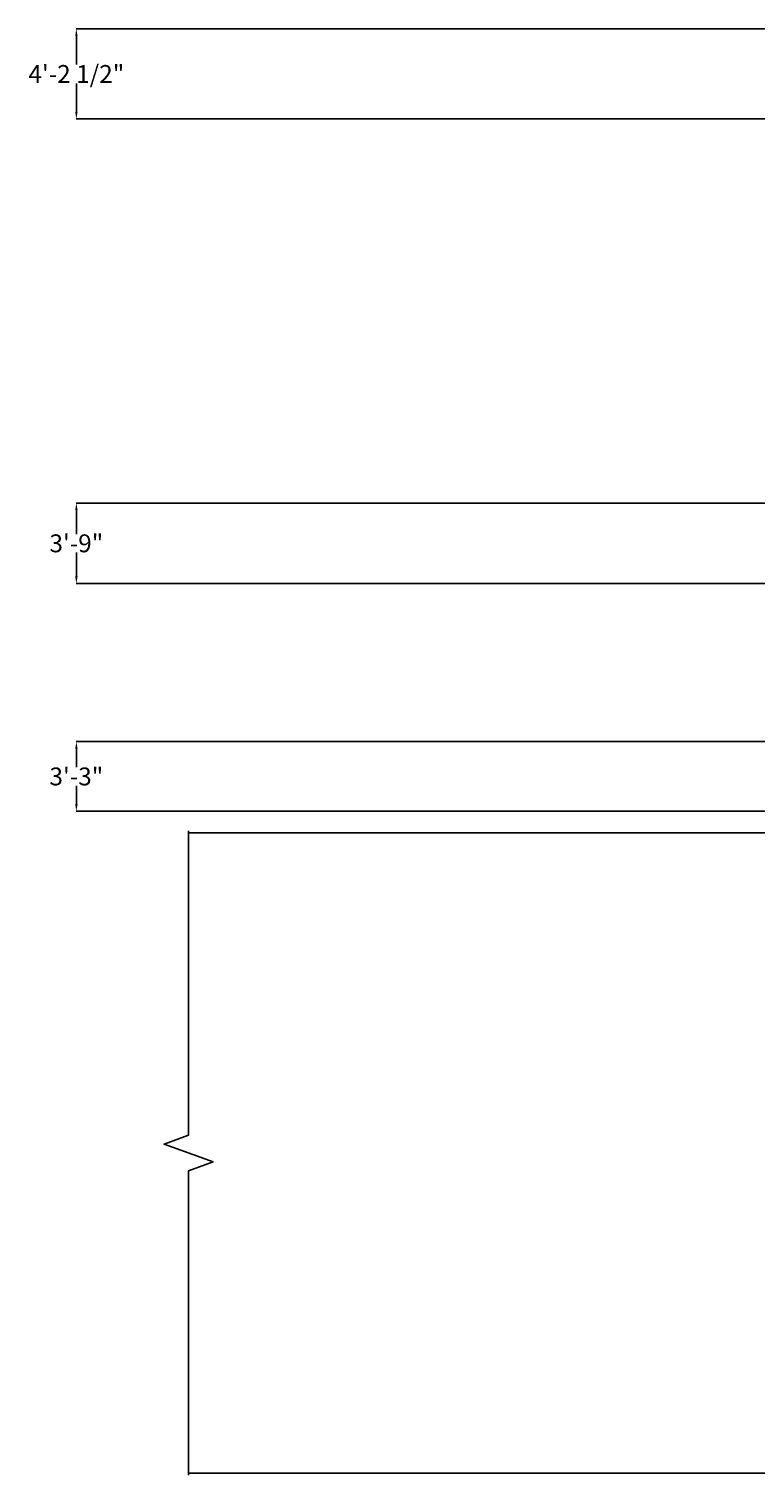
# Model space of a CAD drawing. Units: inches. Extents: x 529 to 1659, y 271 to 1222.
# Tile 1 of 5: x 529 to 936, y 326 to 1136. Entities that reach past the tile are written whole.
import ezdxf

# ---------------------------------------------------------------- set-up
doc = ezdxf.new("R2010")
doc.units = ezdxf.units.IN
doc.header["$MEASUREMENT"] = 0
doc.layers.add('C-ROAD', color=7, linetype='Continuous', lineweight=25)
doc.layers.add('DIM', color=241, linetype='Continuous', lineweight=18)
doc.styles.get("Standard").update_dxf_attribs({"font": 'arial.ttf', "height": 10})
doc.dimstyles.get("Standard").update_dxf_attribs({"dimtxt": 6, "dimasz": 4, "dimexe": 0.18, "dimexo": 0.0625, "dimgap": 0.09, "dimtad": 0, "dimtih": 1, "dimtoh": 1, "dimdec": 0, "dimrnd": 6, "dimzin": 0, "dimdsep": 46, "dimlunit": 3, "dimtxsty": 'Standard', "dimcen": 0.09, "dimadec": 0, "dimazin": 0, "dimtfac": 1, "dimtdec": 0, "dimtofl": 0, "dimtmove": 0, "dimatfit": 3, "dimfxl": 1, "dimtolj": 1, "dimtzin": 0, "dimarcsym": 0})

# ---------------------------------------------------------------- blocks, each defined once
blk = doc.blocks.new('ROAD-BREAKLINE')
blk.add_lwpolyline([(13.74, 0), (13.74, 170.31), (27.47, 175.31), (0, 185.31), (13.74, 190.31), (13.74, 360.62)])
blk = doc.blocks.new('*D32')
at = {"layer": 'Defpoints', "color": 0, "transparency": 16777216}
for p in [(555.49, 736.86), (1020.49, 736.86), (1020.49, 697.86)]:
    blk.add_point(p, dxfattribs=at)
at = {"layer": 'DIM', "color": 0, "lineweight": -2, "transparency": 16777216}
for p, q in [((1020.43, 736.86), (555.31, 736.86)), ((555.49, 732.86), (555.49, 722.55)), ((555.49, 701.86), (555.49, 712.16)), ((1020.43, 697.86), (555.31, 697.86))]:
    blk.add_line(p, q, dxfattribs=at)
at = {"layer": 'DIM', "color": 0, "transparency": 16777216}
for points in [[(554.83, 732.86), (556.16, 732.86), (555.49, 736.86)], [(554.83, 701.86), (556.16, 701.86), (555.49, 697.86)]]:
    blk.add_solid(points, dxfattribs=at)
at = {"layer": 'DIM', "color": 0, "transparency": 16777216, "insert": (555.49, 717.36), "char_height": 10, "attachment_point": 5}
blk.add_mtext('\\A1;3\'-3"', dxfattribs=at)
blk = doc.blocks.new('*D33')
at = {"layer": 'Defpoints', "color": 0, "transparency": 16777216}
for p in [(555.49, 870.44), (1020.49, 870.44), (1020.41, 825.31)]:
    blk.add_point(p, dxfattribs=at)
at = {"layer": 'DIM', "color": 0, "lineweight": -2, "transparency": 16777216}
for p, q in [((1020.43, 870.44), (555.31, 870.44)), ((555.49, 866.44), (555.49, 853.07)), ((555.49, 829.31), (555.49, 842.67)), ((1020.35, 825.31), (555.31, 825.31))]:
    blk.add_line(p, q, dxfattribs=at)
at = {"layer": 'DIM', "color": 0, "transparency": 16777216}
for points in [[(554.83, 866.44), (556.16, 866.44), (555.49, 870.44)], [(554.83, 829.31), (556.16, 829.31), (555.49, 825.31)]]:
    blk.add_solid(points, dxfattribs=at)
at = {"layer": 'DIM', "color": 0, "transparency": 16777216, "insert": (555.49, 847.87), "char_height": 10, "attachment_point": 5}
blk.add_mtext('\\A1;3\'-9"', dxfattribs=at)
blk = doc.blocks.new('*D35')
at = {"layer": 'Defpoints', "color": 0, "transparency": 16777216}
for p in [(555.49, 1135.86), (1020.49, 1135.86), (1029.49, 1085.43)]:
    blk.add_point(p, dxfattribs=at)
at = {"layer": 'DIM', "color": 0, "lineweight": -2, "transparency": 16777216}
for p, q in [((1020.43, 1135.86), (555.31, 1135.86)), ((555.49, 1131.86), (555.49, 1115.9)), ((555.49, 1089.43), (555.49, 1105.38)), ((1029.43, 1085.43), (555.31, 1085.43))]:
    blk.add_line(p, q, dxfattribs=at)
at = {"layer": 'DIM', "color": 0, "transparency": 16777216}
for points in [[(554.83, 1131.86), (556.16, 1131.86), (555.49, 1135.86)], [(554.83, 1089.43), (556.16, 1089.43), (555.49, 1085.43)]]:
    blk.add_solid(points, dxfattribs=at)
at = {"layer": 'DIM', "color": 0, "transparency": 16777216, "insert": (555.49, 1110.64), "char_height": 10, "attachment_point": 5}
blk.add_mtext('\\A1;4\'-2 1/2"', dxfattribs=at)

msp = doc.modelspace()

# ---------------------------------------------------------------- linework, layer by layer
at = {"layer": 'C-ROAD'}
for p, q in [((1567.16, 685.86), (618.33, 685.86)), ((1567.16, 685.86), (618.33, 685.86)), ((1567.16, 327.24), (618.33, 327.24))]:
    msp.add_line(p, q, dxfattribs=at)

# ---------------------------------------------------------------- block references
msp.add_blockref('ROAD-BREAKLINE', (604.59, 326.24), dxfattribs=at)

# ---------------------------------------------------------------- dimensions: what is measured, and where the dimension line sits
at = {"layer": 'DIM'}
for base, p1, p2, picture, middle in [((555.49, 1135.86), (1029.49, 1085.43), (1020.49, 1135.86), '*D35', (555.49, 1110.64)), ((555.49, 870.44), (1020.41, 825.31), (1020.49, 870.44), '*D33', (555.49, 847.87)), ((555.49, 736.86), (1020.49, 697.86), (1020.49, 736.86), '*D32', (555.49, 717.36))]:
    dim = msp.add_linear_dim(base=base, p1=p1, p2=p2, angle=90, dimstyle='Standard', override={"dimdec": 1, "dimlfac": 1, "dimrnd": 0, "dimzin": 1, "dimdsep": 46, "dimlunit": 4, "dimfrac": 2}, dxfattribs=at)
    dim.commit()
    dim.dimension.update_dxf_attribs({"geometry": picture, "text_midpoint": middle})

doc.saveas('drawing.dxf')
